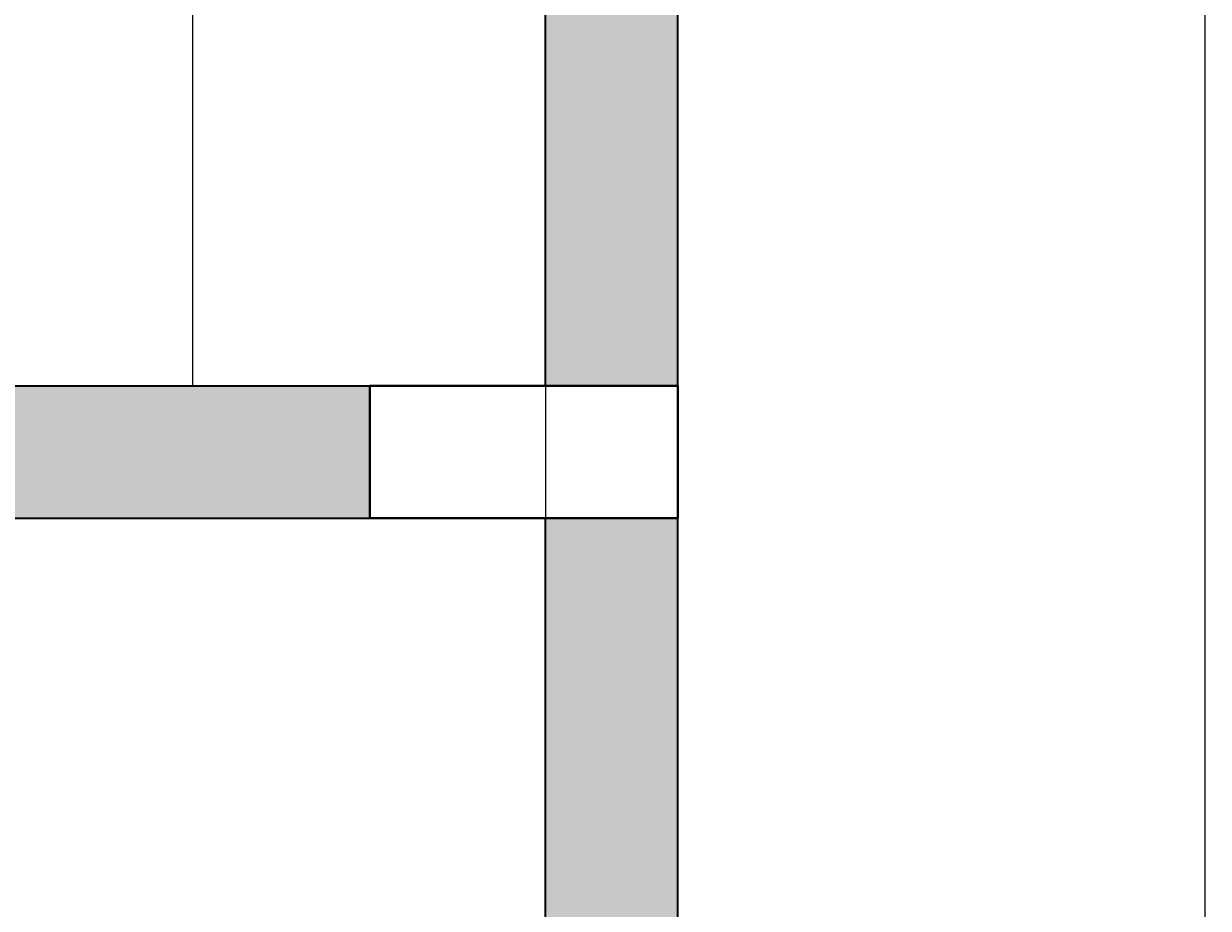
# Model space of a CAD drawing. Units: inches. Extents: x 1568 to 2529, y 2149 to 2897.
# Tile 4 of 16: x 1929 to 2010, y 2304 to 2364. Entities that reach past the tile are written whole.
import ezdxf

# ---------------------------------------------------------------- set-up
doc = ezdxf.new("R2010")
doc.units = ezdxf.units.IN
for name, color, linetype, lineweight in [('A-ANNO-DIMS', 2, 'Continuous', 18), ('A-COLS', 7, 'Continuous', 40), ('A-FLOR-FIXT', 9, 'Continuous', 18), ('A-WALL-PATT', 172, 'Continuous', 13), ('wall', 7, 'Continuous', 35)]:
    doc.layers.add(name, color=color, linetype=linetype, lineweight=lineweight)
doc.styles.get("Standard").update_dxf_attribs({"font": 'arial.ttf'})
doc.dimstyles.get("Standard").update_dxf_attribs({"dimtxt": 0.18, "dimasz": 0.18, "dimexe": 0.18, "dimexo": 0.0625, "dimgap": 0.09, "dimtad": 0, "dimtih": 1, "dimtoh": 1, "dimdec": 4, "dimzin": 0, "dimdsep": 46, "dimtxsty": 'Standard', "dimcen": 0.09, "dimadec": 0, "dimazin": 0, "dimtfac": 1, "dimtdec": 4, "dimtofl": 0, "dimtmove": 0, "dimatfit": 3, "dimfxl": 1, "dimtolj": 1, "dimtzin": 0, "dimarcsym": 0})

# ---------------------------------------------------------------- blocks, each defined once
blk = doc.blocks.new('*D28')
at = {"layer": 'A-ANNO-DIMS', "color": 0, "lineweight": -2, "transparency": 16777216}
for p, q in [((1973.643, 2801.532), (2009.61, 2801.532)), ((2009.43, 2801.352), (2009.43, 2501.714)), ((2009.43, 2201.712), (2009.43, 2501.35)), ((1973.613, 2201.532), (2009.61, 2201.532))]:
    blk.add_line(p, q, dxfattribs=at)
at = {"layer": 'A-ANNO-DIMS', "color": 0, "transparency": 16777216}
for points in [[(2009.4, 2801.352), (2009.46, 2801.352), (2009.43, 2801.532)], [(2009.4, 2201.712), (2009.46, 2201.712), (2009.43, 2201.532)]]:
    blk.add_solid(points, dxfattribs=at)
at = {"layer": 'Defpoints', "color": 0, "transparency": 16777216}
for p in [(1973.58, 2801.532), (2009.43, 2801.532), (1973.551, 2201.532)]:
    blk.add_point(p, dxfattribs=at)
at = {"layer": 'A-ANNO-DIMS', "color": 0, "transparency": 16777216, "insert": (2009.43, 2501.532), "char_height": 0.18, "attachment_point": 5}
blk.add_mtext('\\A1;600', dxfattribs=at)
blk = doc.blocks.new('*D32')
at = {"layer": 'A-ANNO-DIMS', "color": 0, "lineweight": -2, "transparency": 16777216}
for p, q in [((1964.551, 2792.469), (1964.551, 2165.502)), ((1904.551, 2753.401), (1904.551, 2165.502)), ((1904.731, 2165.682), (1934.332, 2165.682)), ((1964.371, 2165.682), (1934.77, 2165.682))]:
    blk.add_line(p, q, dxfattribs=at)
at = {"layer": 'A-ANNO-DIMS', "color": 0, "transparency": 16777216}
for points in [[(1904.731, 2165.712), (1904.731, 2165.652), (1904.551, 2165.682)], [(1964.371, 2165.712), (1964.371, 2165.652), (1964.551, 2165.682)]]:
    blk.add_solid(points, dxfattribs=at)
at = {"layer": 'Defpoints', "color": 0, "transparency": 16777216}
for p in [(1964.551, 2792.532), (1904.551, 2753.463), (1964.551, 2165.682)]:
    blk.add_point(p, dxfattribs=at)
at = {"layer": 'A-ANNO-DIMS', "color": 0, "transparency": 16777216, "insert": (1934.551, 2165.682), "char_height": 0.18, "attachment_point": 5}
blk.add_mtext('\\A1;60', dxfattribs=at)

msp = doc.modelspace()

# ---------------------------------------------------------------- hatches: boundary and pattern name
at = {"layer": 'A-WALL-PATT'}
h = msp.add_hatch(color=256, dxfattribs=at)
h.dxf.hatch_style = 1
h.paths.add_polyline_path([(1738.1593, 2801.532), (1634.4841, 2801.532), (1634.4841, 2792.532), (1738.1593, 2792.532)])
h.paths.add_polyline_path([(1812.4114, 2801.532), (1759.0925, 2801.532), (1759.0925, 2792.532), (1812.4114, 2792.532)])
h.paths.add_polyline_path([(1952.647, 2801.532), (1848.4114, 2801.532), (1848.4114, 2792.532), (1952.647, 2792.532)])
h.paths.add_polyline_path([(1973.5509, 2792.532), (1964.5509, 2792.532), (1964.5509, 2699.1671), (1973.5509, 2699.1671)])
h.paths.add_polyline_path([(1973.5509, 2663.1671), (1964.5509, 2663.1671), (1964.5509, 2630.5978), (1973.5509, 2630.5978)])
h.paths.add_polyline_path([(1973.5509, 2609.6646), (1964.5509, 2609.6646), (1964.5509, 2572.3679), (1973.5509, 2572.3679)])
h.paths.add_polyline_path([(1622.5509, 2753.3576), (1622.3864, 2753.3576), (1613.5509, 2753.3576), (1613.5509, 2705.9172), (1622.5509, 2705.9172)])
h.paths.add_polyline_path([(1622.5509, 2669.9172), (1613.5509, 2669.9172), (1613.5509, 2624.532), (1622.5509, 2624.532)])
h.paths.add_polyline_path([(1759.0509, 2757.9833), (1754.5509, 2757.9833), (1754.5509, 2744.532), (1622.5509, 2744.532), (1622.5509, 2740.032), (1754.5509, 2740.032), (1754.5509, 2730.8156), (1759.0509, 2730.8156), (1759.0509, 2740.032)])
h.paths.add_polyline_path([(1759.0509, 2690.8156), (1754.5509, 2690.8156), (1754.5509, 2624.532), (1759.0509, 2624.532)])
h.paths.add_polyline_path([(1738.1177, 2620.032), (1634.4841, 2620.032), (1634.4841, 2615.532), (1738.1177, 2615.532)])
h.paths.add_polyline_path([(1622.5509, 2615.532), (1613.5509, 2615.532), (1613.5509, 2564.2764), (1622.5509, 2564.2764)])
h.paths.add_polyline_path([(1759.0509, 2411.2271), (1754.5509, 2411.2271), (1754.5509, 2339.532), (1759.0509, 2339.532)])
h.paths.add_polyline_path([(1759.0509, 2464.032), (1734.3925, 2464.032), (1622.5509, 2464.032), (1622.5509, 2459.532), (1736.5509, 2459.532), (1754.5509, 2459.532), (1754.5509, 2451.2271), (1759.0509, 2451.2271)])
h.paths.add_polyline_path([(1844.5509, 2471.532), (1858.1805, 2471.532), (1858.1805, 2476.032), (1844.5509, 2476.032), (1844.5509, 2510.0763), (1840.0509, 2510.0763), (1840.0509, 2476.032), (1840.0509, 2339.532), (1844.5509, 2339.532)])
h.paths.add_polyline_path([(1844.5509, 2596.032), (1964.5509, 2596.032), (1964.5509, 2600.532), (1840.0509, 2600.532), (1840.0509, 2570.0763), (1844.5509, 2570.0763)])
h.paths.add_polyline_path([(1964.5509, 2476.032), (1894.1805, 2476.032), (1894.1805, 2471.532), (1964.5509, 2471.532)])
h.paths.add_polyline_path([(1622.5509, 2528.2764), (1613.5509, 2528.2764), (1613.5509, 2436.512), (1622.5509, 2436.512)])
h.paths.add_polyline_path([(1622.5509, 2400.512), (1613.5509, 2400.512), (1613.5509, 2339.532), (1622.5509, 2339.532)])
h.paths.add_polyline_path([(1738.9144, 2339.532), (1634.4841, 2339.532), (1634.4841, 2330.532), (1738.9144, 2330.532)])
h.paths.add_polyline_path([(1792.463, 2336.532, -0.0187698), (1792.5756, 2339.532), (1783.8928, 2339.532), (1783.8928, 2330.532), (1792.463, 2330.532)])
h.paths.add_polyline_path([(1952.6177, 2339.532), (1885.2912, 2339.532), (1885.2912, 2330.532), (1952.6177, 2330.532)])
h.paths.add_polyline_path([(1973.5509, 2422.371), (1964.5509, 2422.371), (1964.5509, 2395.032), (1964.5509, 2387.286), (1964.5509, 2339.532), (1973.5509, 2339.532)])
h.paths.add_polyline_path([(1973.5509, 2536.3679), (1964.5509, 2536.3679), (1964.5509, 2476.032), (1964.5509, 2458.371), (1973.5509, 2458.371)])
h = msp.add_hatch(color=256, dxfattribs=at)
h.dxf.hatch_style = 1
h.paths.add_polyline_path([(1973.5509, 2330.532), (1964.5509, 2330.532), (1964.5509, 2210.532), (1848.5145, 2210.532), (1848.5145, 2201.532), (1973.5509, 2201.532)])
h.paths.add_polyline_path([(1622.5509, 2330.532), (1613.5509, 2330.532), (1613.5509, 2201.532), (1752.5179, 2201.532), (1752.5179, 2210.532), (1622.5509, 2210.532)])

# ---------------------------------------------------------------- linework, layer by layer
at = {"layer": 'A-COLS'}
msp.add_lwpolyline([(1952.6177, 2339.532), (1973.5509, 2339.532), (1973.5509, 2330.532), (1952.6177, 2330.532)], close=True, dxfattribs=at)
at = {"layer": 'A-FLOR-FIXT'}
msp.add_line((1940.5509, 2471.532), (1940.5509, 2339.532), dxfattribs=at)
at = {"layer": 'wall'}
for p, q in [((1830.713, 2339.532), (1964.5509, 2339.532)), ((1622.5509, 2330.532), (1964.5509, 2330.532))]:
    msp.add_line(p, q, dxfattribs=at)
msp.add_lwpolyline([(1613.5509, 2201.532), (1973.5509, 2201.532), (1973.5509, 2801.532), (1613.5509, 2801.532)], close=True, dxfattribs=at)
for points in [[(1964.5509, 2339.532), (1964.5509, 2390.532)], [(1848.5145, 2210.532), (1964.5509, 2210.532), (1964.5509, 2330.532)]]:
    msp.add_lwpolyline(points, dxfattribs=at)

# ---------------------------------------------------------------- dimensions: what is measured, and where the dimension line sits
at = {"layer": 'A-ANNO-DIMS'}
dim = msp.add_linear_dim(base=(2009.4302, 2801.532), p1=(1973.5509, 2201.532), p2=(1973.5802, 2801.532), angle=90, dimstyle='Standard', override={"dimdec": 0, "dimlfac": 1, "dimrnd": 0, "dimzin": 0, "dimdsep": 46, "dimlunit": 2}, dxfattribs=at)
dim.commit()
dim.dimension.update_dxf_attribs({"geometry": '*D28', "text_midpoint": (2009.4302, 2501.532)})
dim = msp.add_linear_dim(base=(1964.5509, 2165.682), p1=(1904.5509, 2753.4635), p2=(1964.5509, 2792.532), dimstyle='Standard', override={"dimdec": 0, "dimlfac": 1, "dimrnd": 0, "dimzin": 0, "dimdsep": 46, "dimlunit": 2}, dxfattribs=at)
dim.commit()
dim.dimension.update_dxf_attribs({"geometry": '*D32', "text_midpoint": (1934.5509, 2165.682)})

doc.saveas('drawing.dxf')
